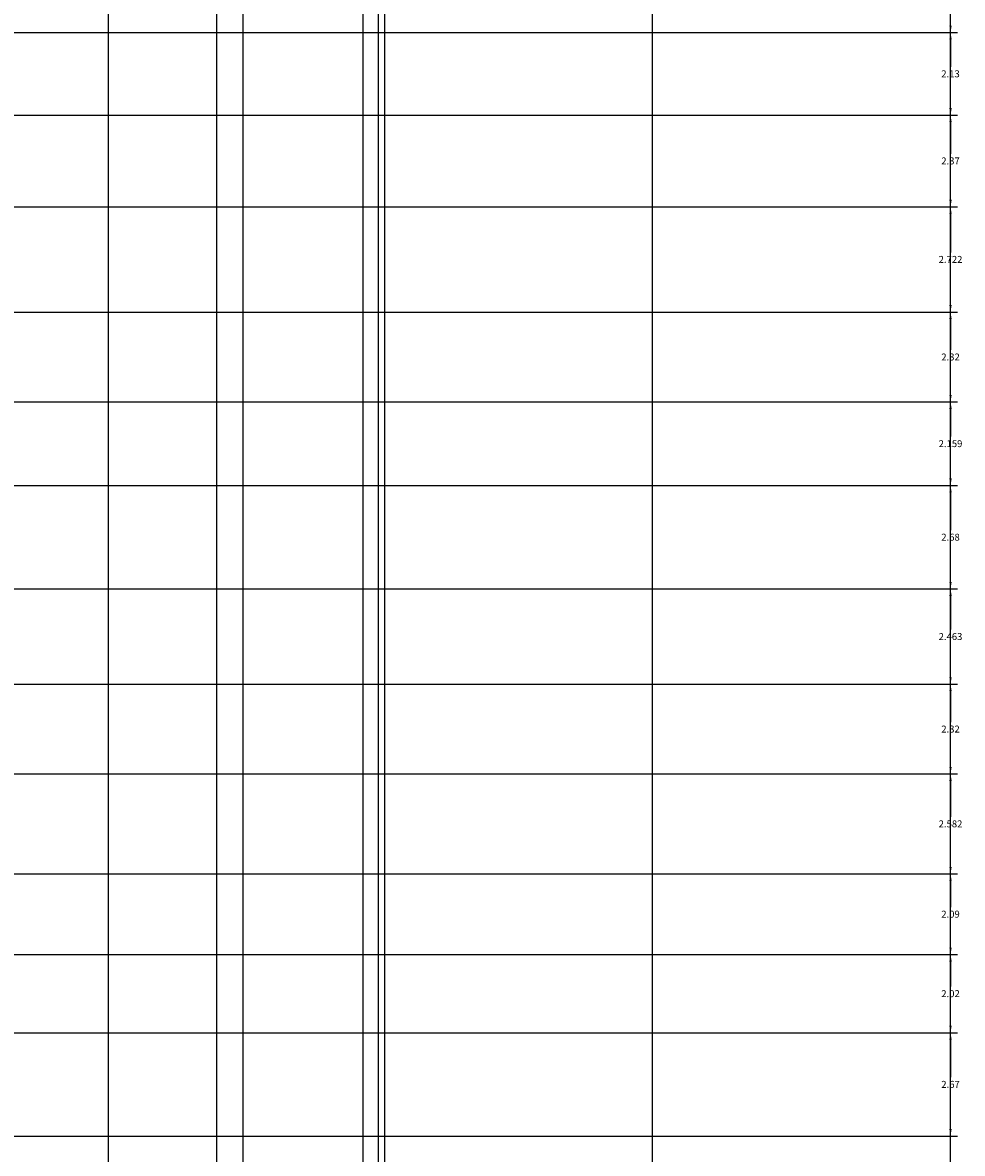
# Model space of a CAD drawing. Units: inches. Extents: x 23 to 132, y 5 to 105.
# Tile 9 of 14: x 105 to 129, y 21 to 50. Entities that reach past the tile are written whole.
import ezdxf

# ---------------------------------------------------------------- set-up
doc = ezdxf.new("R2010")
doc.units = ezdxf.units.IN
doc.header["$MEASUREMENT"] = 0
doc.layers.add('A-ANNO-DIMS', color=2, linetype='Continuous', lineweight=18)
doc.styles.get("Standard").update_dxf_attribs({"font": 'arial.ttf'})
doc.dimstyles.get("Standard").update_dxf_attribs({"dimtxt": 0.18, "dimasz": 0.18, "dimexe": 0.18, "dimexo": 0.0625, "dimgap": 0.09, "dimtad": 0, "dimtih": 1, "dimtoh": 1, "dimdec": 4, "dimzin": 0, "dimdsep": 46, "dimtxsty": 'Standard', "dimcen": 0.09, "dimadec": 0, "dimazin": 0, "dimtfac": 1, "dimtdec": 4, "dimtofl": 0, "dimtmove": 0, "dimatfit": 3, "dimfxl": 1, "dimtolj": 1, "dimtzin": 0, "dimarcsym": 0})

# ---------------------------------------------------------------- blocks, each defined once
blk = doc.blocks.new('*D3')
at = {"layer": 'A-ANNO-DIMS', "color": 0, "lineweight": -2, "transparency": 16777216}
for p, q in [((121.409, 99.285), (129.239, 99.285)), ((129.059, 99.105), (129.059, 55.423)), ((129.059, 11.378), (129.059, 55.06)), ((72.981, 11.198), (129.239, 11.198))]:
    blk.add_line(p, q, dxfattribs=at)
at = {"layer": 'A-ANNO-DIMS', "color": 0, "transparency": 16777216}
for points in [[(129.029, 99.105), (129.089, 99.105), (129.059, 99.285)], [(129.029, 11.378), (129.089, 11.378), (129.059, 11.198)]]:
    blk.add_solid(points, dxfattribs=at)
at = {"layer": 'Defpoints', "color": 0, "transparency": 16777216}
for p in [(121.346, 99.285), (129.059, 99.285), (72.919, 11.198)]:
    blk.add_point(p, dxfattribs=at)
at = {"layer": 'A-ANNO-DIMS', "color": 0, "transparency": 16777216, "insert": (129.059, 55.241), "char_height": 0.18, "attachment_point": 5}
blk.add_mtext('\\A1;88.09', dxfattribs=at)
blk = doc.blocks.new('*D35')
at = {"layer": 'A-ANNO-DIMS', "color": 0, "lineweight": -2, "transparency": 16777216}
for p, q in [((83.576, 52.617), (129.239, 52.617)), ((129.059, 52.437), (129.059, 51.532)), ((129.059, 50.264), (129.059, 51.168)), ((83.576, 50.084), (129.239, 50.084))]:
    blk.add_line(p, q, dxfattribs=at)
at = {"layer": 'A-ANNO-DIMS', "color": 0, "transparency": 16777216}
for points in [[(129.029, 52.437), (129.089, 52.437), (129.059, 52.617)], [(129.029, 50.264), (129.089, 50.264), (129.059, 50.084)]]:
    blk.add_solid(points, dxfattribs=at)
at = {"layer": 'Defpoints', "color": 0, "transparency": 16777216}
for p in [(83.514, 52.617), (83.514, 50.084), (129.059, 50.084)]:
    blk.add_point(p, dxfattribs=at)
at = {"layer": 'A-ANNO-DIMS', "color": 0, "transparency": 16777216, "insert": (129.059, 51.35), "char_height": 0.18, "attachment_point": 5}
blk.add_mtext('\\A1;2.53', dxfattribs=at)
blk = doc.blocks.new('*D36')
at = {"layer": 'A-ANNO-DIMS', "color": 0, "lineweight": -2, "transparency": 16777216}
for p, q in [((83.576, 50.084), (129.239, 50.084)), ((129.059, 49.904), (129.059, 49.198)), ((129.059, 48.129), (129.059, 48.834)), ((83.576, 47.949), (129.239, 47.949))]:
    blk.add_line(p, q, dxfattribs=at)
at = {"layer": 'A-ANNO-DIMS', "color": 0, "transparency": 16777216}
for points in [[(129.029, 49.904), (129.089, 49.904), (129.059, 50.084)], [(129.029, 48.129), (129.089, 48.129), (129.059, 47.949)]]:
    blk.add_solid(points, dxfattribs=at)
at = {"layer": 'Defpoints', "color": 0, "transparency": 16777216}
for p in [(83.514, 50.084), (83.514, 47.949), (129.059, 47.949)]:
    blk.add_point(p, dxfattribs=at)
at = {"layer": 'A-ANNO-DIMS', "color": 0, "transparency": 16777216, "insert": (129.059, 49.016), "char_height": 0.18, "attachment_point": 5}
blk.add_mtext('\\A1;2.13', dxfattribs=at)
blk = doc.blocks.new('*D37')
at = {"layer": 'A-ANNO-DIMS', "color": 0, "lineweight": -2, "transparency": 16777216}
for p, q in [((83.576, 47.949), (129.239, 47.949)), ((129.059, 47.769), (129.059, 46.946)), ((129.059, 45.759), (129.059, 46.582)), ((83.576, 45.579), (129.239, 45.579))]:
    blk.add_line(p, q, dxfattribs=at)
at = {"layer": 'A-ANNO-DIMS', "color": 0, "transparency": 16777216}
for points in [[(129.029, 47.769), (129.089, 47.769), (129.059, 47.949)], [(129.029, 45.759), (129.089, 45.759), (129.059, 45.579)]]:
    blk.add_solid(points, dxfattribs=at)
at = {"layer": 'Defpoints', "color": 0, "transparency": 16777216}
for p in [(83.514, 47.949), (83.514, 45.579), (129.059, 45.579)]:
    blk.add_point(p, dxfattribs=at)
at = {"layer": 'A-ANNO-DIMS', "color": 0, "transparency": 16777216, "insert": (129.059, 46.764), "char_height": 0.18, "attachment_point": 5}
blk.add_mtext('\\A1;2.37', dxfattribs=at)
blk = doc.blocks.new('*D38')
at = {"layer": 'A-ANNO-DIMS', "color": 0, "lineweight": -2, "transparency": 16777216}
for p, q in [((83.576, 45.579), (129.239, 45.579)), ((129.059, 45.399), (129.059, 44.398)), ((129.059, 43.037), (129.059, 44.037)), ((83.576, 42.857), (129.239, 42.857))]:
    blk.add_line(p, q, dxfattribs=at)
at = {"layer": 'A-ANNO-DIMS', "color": 0, "transparency": 16777216}
for points in [[(129.029, 45.399), (129.089, 45.399), (129.059, 45.579)], [(129.029, 43.037), (129.089, 43.037), (129.059, 42.857)]]:
    blk.add_solid(points, dxfattribs=at)
at = {"layer": 'Defpoints', "color": 0, "transparency": 16777216}
for p in [(83.514, 45.579), (83.514, 42.857), (129.059, 42.857)]:
    blk.add_point(p, dxfattribs=at)
at = {"layer": 'A-ANNO-DIMS', "color": 0, "transparency": 16777216, "insert": (129.059, 44.218), "char_height": 0.18, "attachment_point": 5}
blk.add_mtext('\\A1;2.722', dxfattribs=at)
blk = doc.blocks.new('*D39')
at = {"layer": 'A-ANNO-DIMS', "color": 0, "lineweight": -2, "transparency": 16777216}
for p, q in [((83.576, 42.857), (129.239, 42.857)), ((129.059, 42.677), (129.059, 41.877)), ((129.059, 40.714), (129.059, 41.513)), ((83.576, 40.534), (129.239, 40.534))]:
    blk.add_line(p, q, dxfattribs=at)
at = {"layer": 'A-ANNO-DIMS', "color": 0, "transparency": 16777216}
for points in [[(129.029, 42.677), (129.089, 42.677), (129.059, 42.857)], [(129.029, 40.714), (129.089, 40.714), (129.059, 40.534)]]:
    blk.add_solid(points, dxfattribs=at)
at = {"layer": 'Defpoints', "color": 0, "transparency": 16777216}
for p in [(83.514, 42.857), (83.514, 40.534), (129.059, 40.534)]:
    blk.add_point(p, dxfattribs=at)
at = {"layer": 'A-ANNO-DIMS', "color": 0, "transparency": 16777216, "insert": (129.059, 41.695), "char_height": 0.18, "attachment_point": 5}
blk.add_mtext('\\A1;2.32', dxfattribs=at)
blk = doc.blocks.new('*D40')
at = {"layer": 'A-ANNO-DIMS', "color": 0, "lineweight": -2, "transparency": 16777216}
for p, q in [((83.576, 40.534), (129.239, 40.534)), ((129.059, 40.354), (129.059, 39.637)), ((129.059, 38.555), (129.059, 39.273)), ((83.576, 38.375), (129.239, 38.375))]:
    blk.add_line(p, q, dxfattribs=at)
at = {"layer": 'A-ANNO-DIMS', "color": 0, "transparency": 16777216}
for points in [[(129.029, 40.354), (129.089, 40.354), (129.059, 40.534)], [(129.029, 38.555), (129.089, 38.555), (129.059, 38.375)]]:
    blk.add_solid(points, dxfattribs=at)
at = {"layer": 'Defpoints', "color": 0, "transparency": 16777216}
for p in [(83.514, 40.534), (83.514, 38.375), (129.059, 38.375)]:
    blk.add_point(p, dxfattribs=at)
at = {"layer": 'A-ANNO-DIMS', "color": 0, "transparency": 16777216, "insert": (129.059, 39.455), "char_height": 0.18, "attachment_point": 5}
blk.add_mtext('\\A1;2.159', dxfattribs=at)
blk = doc.blocks.new('*D41')
at = {"layer": 'A-ANNO-DIMS', "color": 0, "lineweight": -2, "transparency": 16777216}
for p, q in [((83.576, 38.375), (129.239, 38.375)), ((129.059, 38.195), (129.059, 37.219)), ((129.059, 35.88), (129.059, 36.856)), ((83.576, 35.7), (129.239, 35.7))]:
    blk.add_line(p, q, dxfattribs=at)
at = {"layer": 'A-ANNO-DIMS', "color": 0, "transparency": 16777216}
for points in [[(129.029, 38.195), (129.089, 38.195), (129.059, 38.375)], [(129.029, 35.88), (129.089, 35.88), (129.059, 35.7)]]:
    blk.add_solid(points, dxfattribs=at)
at = {"layer": 'Defpoints', "color": 0, "transparency": 16777216}
for p in [(83.514, 38.375), (83.514, 35.7), (129.059, 35.7)]:
    blk.add_point(p, dxfattribs=at)
at = {"layer": 'A-ANNO-DIMS', "color": 0, "transparency": 16777216, "insert": (129.059, 37.037), "char_height": 0.18, "attachment_point": 5}
blk.add_mtext('\\A1;2.68', dxfattribs=at)
blk = doc.blocks.new('*D42')
at = {"layer": 'A-ANNO-DIMS', "color": 0, "lineweight": -2, "transparency": 16777216}
for p, q in [((83.576, 35.7), (129.239, 35.7)), ((129.059, 35.52), (129.059, 34.65)), ((129.059, 33.417), (129.059, 34.286)), ((83.576, 33.237), (129.239, 33.237))]:
    blk.add_line(p, q, dxfattribs=at)
at = {"layer": 'A-ANNO-DIMS', "color": 0, "transparency": 16777216}
for points in [[(129.029, 35.52), (129.089, 35.52), (129.059, 35.7)], [(129.029, 33.417), (129.089, 33.417), (129.059, 33.237)]]:
    blk.add_solid(points, dxfattribs=at)
at = {"layer": 'Defpoints', "color": 0, "transparency": 16777216}
for p in [(83.514, 35.7), (83.514, 33.237), (129.059, 33.237)]:
    blk.add_point(p, dxfattribs=at)
at = {"layer": 'A-ANNO-DIMS', "color": 0, "transparency": 16777216, "insert": (129.059, 34.468), "char_height": 0.18, "attachment_point": 5}
blk.add_mtext('\\A1;2.463', dxfattribs=at)
blk = doc.blocks.new('*D43')
at = {"layer": 'A-ANNO-DIMS', "color": 0, "lineweight": -2, "transparency": 16777216}
for p, q in [((83.576, 33.237), (129.239, 33.237)), ((129.059, 33.057), (129.059, 32.259)), ((129.059, 31.097), (129.059, 31.895)), ((83.576, 30.917), (129.239, 30.917))]:
    blk.add_line(p, q, dxfattribs=at)
at = {"layer": 'A-ANNO-DIMS', "color": 0, "transparency": 16777216}
for points in [[(129.029, 33.057), (129.089, 33.057), (129.059, 33.237)], [(129.029, 31.097), (129.089, 31.097), (129.059, 30.917)]]:
    blk.add_solid(points, dxfattribs=at)
at = {"layer": 'Defpoints', "color": 0, "transparency": 16777216}
for p in [(83.514, 33.237), (83.514, 30.917), (129.059, 30.917)]:
    blk.add_point(p, dxfattribs=at)
at = {"layer": 'A-ANNO-DIMS', "color": 0, "transparency": 16777216, "insert": (129.059, 32.077), "char_height": 0.18, "attachment_point": 5}
blk.add_mtext('\\A1;2.32', dxfattribs=at)
blk = doc.blocks.new('*D44')
at = {"layer": 'A-ANNO-DIMS', "color": 0, "lineweight": -2, "transparency": 16777216}
for p, q in [((83.576, 30.917), (129.239, 30.917)), ((129.059, 30.737), (129.059, 29.808)), ((129.059, 28.515), (129.059, 29.444)), ((83.576, 28.335), (129.239, 28.335))]:
    blk.add_line(p, q, dxfattribs=at)
at = {"layer": 'A-ANNO-DIMS', "color": 0, "transparency": 16777216}
for points in [[(129.029, 30.737), (129.089, 30.737), (129.059, 30.917)], [(129.029, 28.515), (129.089, 28.515), (129.059, 28.335)]]:
    blk.add_solid(points, dxfattribs=at)
at = {"layer": 'Defpoints', "color": 0, "transparency": 16777216}
for p in [(83.514, 30.917), (83.514, 28.335), (129.059, 28.335)]:
    blk.add_point(p, dxfattribs=at)
at = {"layer": 'A-ANNO-DIMS', "color": 0, "transparency": 16777216, "insert": (129.059, 29.626), "char_height": 0.18, "attachment_point": 5}
blk.add_mtext('\\A1;2.582', dxfattribs=at)
blk = doc.blocks.new('*D45')
at = {"layer": 'A-ANNO-DIMS', "color": 0, "lineweight": -2, "transparency": 16777216}
for p, q in [((83.576, 28.335), (129.239, 28.335)), ((129.059, 28.155), (129.059, 27.473)), ((129.059, 26.427), (129.059, 27.109)), ((83.576, 26.247), (129.239, 26.247))]:
    blk.add_line(p, q, dxfattribs=at)
at = {"layer": 'A-ANNO-DIMS', "color": 0, "transparency": 16777216}
for points in [[(129.029, 28.155), (129.089, 28.155), (129.059, 28.335)], [(129.029, 26.427), (129.089, 26.427), (129.059, 26.247)]]:
    blk.add_solid(points, dxfattribs=at)
at = {"layer": 'Defpoints', "color": 0, "transparency": 16777216}
for p in [(83.514, 28.335), (83.514, 26.247), (129.059, 26.247)]:
    blk.add_point(p, dxfattribs=at)
at = {"layer": 'A-ANNO-DIMS', "color": 0, "transparency": 16777216, "insert": (129.059, 27.291), "char_height": 0.18, "attachment_point": 5}
blk.add_mtext('\\A1;2.09', dxfattribs=at)
blk = doc.blocks.new('*D46')
at = {"layer": 'A-ANNO-DIMS', "color": 0, "lineweight": -2, "transparency": 16777216}
for p, q in [((83.576, 26.247), (129.239, 26.247)), ((129.059, 26.067), (129.059, 25.419)), ((129.059, 24.408), (129.059, 25.055)), ((83.576, 24.228), (129.239, 24.228))]:
    blk.add_line(p, q, dxfattribs=at)
at = {"layer": 'A-ANNO-DIMS', "color": 0, "transparency": 16777216}
for points in [[(129.029, 26.067), (129.089, 26.067), (129.059, 26.247)], [(129.029, 24.408), (129.089, 24.408), (129.059, 24.228)]]:
    blk.add_solid(points, dxfattribs=at)
at = {"layer": 'Defpoints', "color": 0, "transparency": 16777216}
for p in [(83.514, 26.247), (83.514, 24.228), (129.059, 24.228)]:
    blk.add_point(p, dxfattribs=at)
at = {"layer": 'A-ANNO-DIMS', "color": 0, "transparency": 16777216, "insert": (129.059, 25.237), "char_height": 0.18, "attachment_point": 5}
blk.add_mtext('\\A1;2.02', dxfattribs=at)
blk = doc.blocks.new('*D47')
at = {"layer": 'A-ANNO-DIMS', "color": 0, "lineweight": -2, "transparency": 16777216}
for p, q in [((83.576, 24.228), (129.239, 24.228)), ((129.059, 24.048), (129.059, 23.074)), ((129.059, 21.737), (129.059, 22.71)), ((83.576, 21.557), (129.239, 21.557))]:
    blk.add_line(p, q, dxfattribs=at)
at = {"layer": 'A-ANNO-DIMS', "color": 0, "transparency": 16777216}
for points in [[(129.029, 24.048), (129.089, 24.048), (129.059, 24.228)], [(129.029, 21.737), (129.089, 21.737), (129.059, 21.557)]]:
    blk.add_solid(points, dxfattribs=at)
at = {"layer": 'Defpoints', "color": 0, "transparency": 16777216}
for p in [(83.514, 24.228), (83.514, 21.557), (129.059, 21.557)]:
    blk.add_point(p, dxfattribs=at)
at = {"layer": 'A-ANNO-DIMS', "color": 0, "transparency": 16777216, "insert": (129.059, 22.892), "char_height": 0.18, "attachment_point": 5}
blk.add_mtext('\\A1;2.67', dxfattribs=at)
blk = doc.blocks.new('*D75')
at = {"layer": 'A-ANNO-DIMS', "color": 0, "lineweight": -2, "transparency": 16777216}
for p, q in [((107.287, 59.528), (107.287, 5.443)), ((110.768, 59.503), (110.768, 5.443)), ((107.467, 5.623), (108.704, 5.623)), ((110.588, 5.623), (109.351, 5.623))]:
    blk.add_line(p, q, dxfattribs=at)
at = {"layer": 'A-ANNO-DIMS', "color": 0, "transparency": 16777216}
for points in [[(107.467, 5.653), (107.467, 5.593), (107.287, 5.623)], [(110.588, 5.653), (110.588, 5.593), (110.768, 5.623)]]:
    blk.add_solid(points, dxfattribs=at)
at = {"layer": 'Defpoints', "color": 0, "transparency": 16777216}
for p in [(107.287, 59.59), (110.768, 59.566), (110.768, 5.623)]:
    blk.add_point(p, dxfattribs=at)
at = {"layer": 'A-ANNO-DIMS', "color": 0, "transparency": 16777216, "insert": (109.028, 5.623), "char_height": 0.18, "attachment_point": 5}
blk.add_mtext('\\A1;3.48', dxfattribs=at)
blk = doc.blocks.new('*D76')
at = {"layer": 'A-ANNO-DIMS', "color": 0, "lineweight": -2, "transparency": 16777216}
for p, q in [((110.768, 59.503), (110.768, 5.443)), ((114.434, 59.528), (114.434, 5.443)), ((110.948, 5.623), (112.207, 5.623)), ((114.254, 5.623), (112.994, 5.623))]:
    blk.add_line(p, q, dxfattribs=at)
at = {"layer": 'A-ANNO-DIMS', "color": 0, "transparency": 16777216}
for points in [[(110.948, 5.653), (110.948, 5.593), (110.768, 5.623)], [(114.254, 5.653), (114.254, 5.593), (114.434, 5.623)]]:
    blk.add_solid(points, dxfattribs=at)
at = {"layer": 'Defpoints', "color": 0, "transparency": 16777216}
for p in [(110.768, 59.566), (114.434, 59.59), (114.434, 5.623)]:
    blk.add_point(p, dxfattribs=at)
at = {"layer": 'A-ANNO-DIMS', "color": 0, "transparency": 16777216, "insert": (112.601, 5.623), "char_height": 0.18, "attachment_point": 5}
blk.add_mtext('\\A1;3.666', dxfattribs=at)
blk = doc.blocks.new('*D91')
at = {"layer": 'A-ANNO-DIMS', "color": 0, "lineweight": -2, "transparency": 16777216}
for p, q in [((110.089, 79.853), (110.089, 5.443)), ((113.872, 79.853), (113.872, 5.443)), ((110.269, 5.623), (111.587, 5.623)), ((113.692, 5.623), (112.374, 5.623))]:
    blk.add_line(p, q, dxfattribs=at)
at = {"layer": 'A-ANNO-DIMS', "color": 0, "transparency": 16777216}
for points in [[(110.269, 5.653), (110.269, 5.593), (110.089, 5.623)], [(113.692, 5.653), (113.692, 5.593), (113.872, 5.623)]]:
    blk.add_solid(points, dxfattribs=at)
at = {"layer": 'Defpoints', "color": 0, "transparency": 16777216}
for p in [(110.089, 79.916), (113.872, 79.916), (113.872, 5.623)]:
    blk.add_point(p, dxfattribs=at)
at = {"layer": 'A-ANNO-DIMS', "color": 0, "transparency": 16777216, "insert": (111.981, 5.623), "char_height": 0.18, "attachment_point": 5}
blk.add_mtext('\\A1;3.783', dxfattribs=at)
blk = doc.blocks.new('*D93')
at = {"layer": 'A-ANNO-DIMS', "color": 0, "lineweight": -2, "transparency": 16777216}
for p, q in [((114.269, 94.721), (114.269, 5.443)), ((121.346, 94.721), (121.346, 5.443)), ((114.449, 5.623), (117.415, 5.623)), ((121.166, 5.623), (118.201, 5.623))]:
    blk.add_line(p, q, dxfattribs=at)
at = {"layer": 'A-ANNO-DIMS', "color": 0, "transparency": 16777216}
for points in [[(114.449, 5.653), (114.449, 5.593), (114.269, 5.623)], [(121.166, 5.653), (121.166, 5.593), (121.346, 5.623)]]:
    blk.add_solid(points, dxfattribs=at)
at = {"layer": 'Defpoints', "color": 0, "transparency": 16777216}
for p in [(114.269, 94.783), (121.346, 94.783), (121.346, 5.623)]:
    blk.add_point(p, dxfattribs=at)
at = {"layer": 'A-ANNO-DIMS', "color": 0, "transparency": 16777216, "insert": (117.808, 5.623), "char_height": 0.18, "attachment_point": 5}
blk.add_mtext('\\A1;7.077', dxfattribs=at)

msp = doc.modelspace()

# ---------------------------------------------------------------- dimensions: what is measured, and where the dimension line sits
at = {"layer": 'A-ANNO-DIMS'}
for base, p1, p2, override, picture, middle in [((129.0589, 99.2846), (72.9188, 11.1983), (121.3461, 99.2846), {"dimdec": 2, "dimlfac": 1, "dimrnd": 0, "dimzin": 0, "dimdsep": 46, "dimlunit": 2}, '*D3', (129.0589, 55.2415)), ((129.0589, 50.0837), (83.5136, 52.6172), (83.5136, 50.0837), {"dimdec": 2, "dimlfac": 1, "dimrnd": 0, "dimzin": 0, "dimdsep": 46, "dimlunit": 2}, '*D35', (129.0589, 51.3504)), ((129.0589, 47.949), (83.5136, 50.0837), (83.5136, 47.949), {"dimdec": 2, "dimlfac": 1, "dimrnd": 0, "dimzin": 0, "dimdsep": 46, "dimlunit": 2}, '*D36', (129.0589, 49.0163)), ((129.0589, 45.5785), (83.5136, 47.949), (83.5136, 45.5785), {"dimdec": 2, "dimlfac": 1, "dimrnd": 0, "dimzin": 0, "dimdsep": 46, "dimlunit": 2}, '*D37', (129.0589, 46.7637)), ((129.0589, 42.8565), (83.5136, 45.5785), (83.5136, 42.8565), {"dimdec": 3, "dimlfac": 1, "dimrnd": 0, "dimzin": 0, "dimdsep": 46, "dimlunit": 2}, '*D38', (129.0589, 44.2175)), ((129.0589, 40.5342), (83.5136, 42.8565), (83.5136, 40.5342), {"dimdec": 2, "dimlfac": 1, "dimrnd": 0, "dimzin": 0, "dimdsep": 46, "dimlunit": 2}, '*D39', (129.0589, 41.6954)), ((129.0589, 38.3751), (83.5136, 40.5342), (83.5136, 38.3751), {"dimdec": 3, "dimlfac": 1, "dimrnd": 0, "dimzin": 0, "dimdsep": 46, "dimlunit": 2}, '*D40', (129.0589, 39.4546)), ((129.0589, 35.6998), (83.5136, 38.3751), (83.5136, 35.6998), {"dimdec": 2, "dimlfac": 1, "dimrnd": 0, "dimzin": 0, "dimdsep": 46, "dimlunit": 2}, '*D41', (129.0589, 37.0375)), ((129.0589, 33.2368), (83.5136, 35.6998), (83.5136, 33.2368), {"dimdec": 3, "dimlfac": 1, "dimrnd": 0, "dimzin": 0, "dimdsep": 46, "dimlunit": 2}, '*D42', (129.0589, 34.4683)), ((129.0589, 30.917), (83.5136, 33.2368), (83.5136, 30.917), {"dimdec": 2, "dimlfac": 1, "dimrnd": 0, "dimzin": 0, "dimdsep": 46, "dimlunit": 2}, '*D43', (129.0589, 32.0769)), ((129.0589, 28.3352), (83.5136, 30.917), (83.5136, 28.3352), {"dimdec": 3, "dimlfac": 1, "dimrnd": 0, "dimzin": 0, "dimdsep": 46, "dimlunit": 2}, '*D44', (129.0589, 29.6261)), ((129.0589, 26.2465), (83.5136, 28.3352), (83.5136, 26.2465), {"dimdec": 2, "dimlfac": 1, "dimrnd": 0, "dimzin": 0, "dimdsep": 46, "dimlunit": 2}, '*D45', (129.0589, 27.2909)), ((129.0589, 24.2279), (83.5136, 26.2465), (83.5136, 24.2279), {"dimdec": 2, "dimlfac": 1, "dimrnd": 0, "dimzin": 0, "dimdsep": 46, "dimlunit": 2}, '*D46', (129.0589, 25.2372)), ((129.0589, 21.5566), (83.5136, 24.2279), (83.5136, 21.5566), {"dimdec": 2, "dimlfac": 1, "dimrnd": 0, "dimzin": 0, "dimdsep": 46, "dimlunit": 2}, '*D47', (129.0589, 22.8923))]:
    dim = msp.add_linear_dim(base=base, p1=p1, p2=p2, angle=90, dimstyle='Standard', override=override, dxfattribs=at)
    dim.commit()
    dim.dimension.update_dxf_attribs({"geometry": picture, "text_midpoint": middle})
for base, p1, p2, override, picture, middle in [((121.3461, 5.6233), (114.2693, 94.7833), (121.3461, 94.7833), {"dimdec": 3, "dimlfac": 1, "dimrnd": 0, "dimzin": 0, "dimdsep": 46, "dimlunit": 2}, '*D93', (117.8077, 5.6233)), ((113.8719, 5.6233), (110.0892, 79.9158), (113.8719, 79.9158), {"dimdec": 3, "dimlfac": 1, "dimrnd": 0, "dimzin": 0, "dimdsep": 46, "dimlunit": 2}, '*D91', (111.9805, 5.6233)), ((110.7677, 5.6233), (107.2874, 59.5904), (110.7677, 59.566), {"dimdec": 2, "dimlfac": 1, "dimrnd": 0, "dimzin": 0, "dimdsep": 46, "dimlunit": 2}, '*D75', (109.0275, 5.6233)), ((114.434, 5.6233), (110.7677, 59.566), (114.434, 59.5904), {"dimdec": 3, "dimlfac": 1, "dimrnd": 0, "dimzin": 0, "dimdsep": 46, "dimlunit": 2}, '*D76', (112.6009, 5.6233))]:
    dim = msp.add_linear_dim(base=base, p1=p1, p2=p2, dimstyle='Standard', override=override, dxfattribs=at)
    dim.commit()
    dim.dimension.update_dxf_attribs({"geometry": picture, "text_midpoint": middle})

doc.saveas('drawing.dxf')
